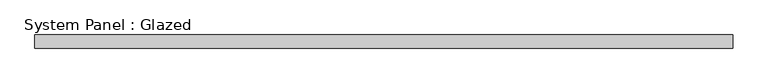
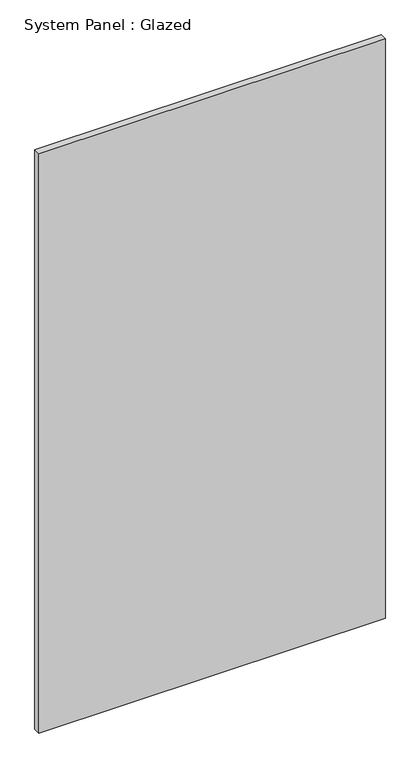
"""IFC4 building model written with IfcOpenShell, lengths in millimetres: plate geometry, System Panel : Glazed."""

from ifc_helpers import new_model, si_unit, origin, origin_with_axes, place, context, project, spatial, polyline, outline, extrude, source, transform, mapped, element, save


def system_panel_glazed_17617b93(model_context):
    return source(origin(), model_context, "Body", "SweptSolid", [
        extrude(outline(polyline([(654.05, 19.05), (-654.05, 19.05), (-654.05, 44.45), (654.05, 44.45), (654.05, 19.05)])), origin_with_axes(), (0.0, 0.0, 1.0), 2311.4),
    ])


if __name__ == "__main__":
    model = new_model("IFC4")
    model_context = context("Model", 3, world=origin())
    ifc_project = project(units=[si_unit("LENGTHUNIT", "METRE", prefix="MILLI")], contexts=[model_context])
    site = spatial("IfcSite", under=ifc_project)
    building = spatial("IfcBuilding", under=site)
    placement = place(None, origin())
    system_panel_glazed_shape = system_panel_glazed_17617b93(model_context)
    element("IfcPlate", 1, ObjectType="System Panel : Glazed", at=placement, inside=building, context=model_context, shape_type="MappedRepresentation", body=[
        mapped(system_panel_glazed_shape, transform((0.0, 0.0, 0.0), x_axis=(1.0, 0.0, 0.0), y_axis=(0.0, 1.0, 0.0), z_axis=(0.0, 0.0, 1.0))),
    ])
    save(model, "model.ifc")

# Revit data of these elements
# Type "System Panel : Glazed"
#   Construction Type Id = "GSP4R"
#   Analytic Construction = "1/8 in Pilkington single glazing"
#   Visual Light Transmittance = 0.9
#   Solar Heat Gain Coefficient = 0.86
#   Heat Transfer Coefficient (U) = 1.18115 BTU/(h·ft²·°F)
# Element 1 (IfcPlate, "System Panel : Glazed")
#   Materials on its faces: "Glass"
# Materials
#   "Glass": class "Glass", colour RGB 0 128 192, transparency 0.75, Description = "Soda Lime Glass", Cost = 0
